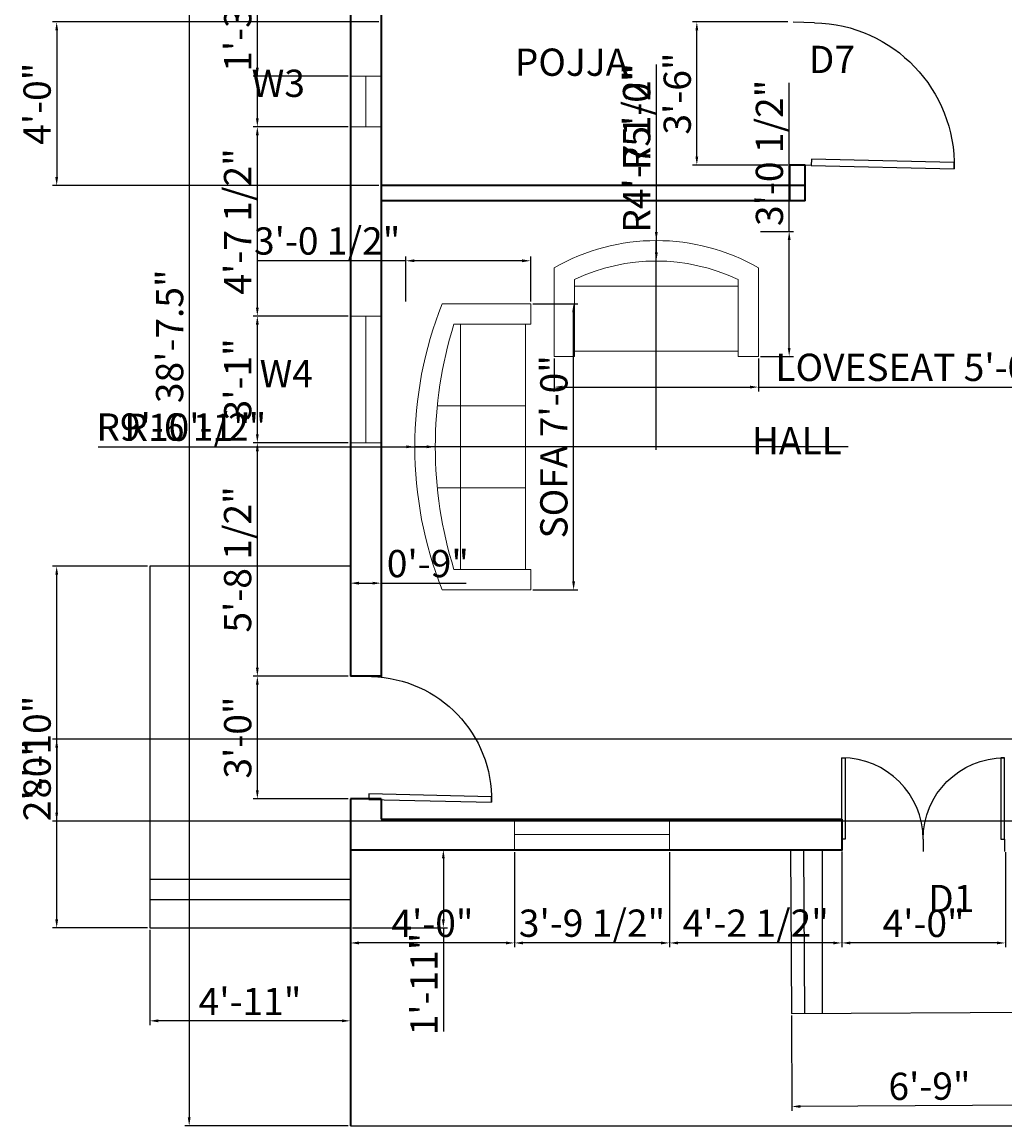
# Model space of a CAD drawing. Units: inches. Extents: x 56 to 631, y 587 to 1198.
# Tile 1 of 3: x 56 to 344, y 622 to 946. Entities that reach past the tile are written whole.
import ezdxf

# ---------------------------------------------------------------- set-up
doc = ezdxf.new("R2010")
doc.units = ezdxf.units.IN
for name, color, linetype, lineweight in [('A-ANNO-DIMS', 2, 'Continuous', 18), ('A-ANNO-TEXT', 7, 'Continuous', 18), ('A-AREA-IDEN', 7, 'Continuous', 25), ('A-DOOR', 3, 'Continuous', 25), ('A-FLOR-OTLN', 7, 'Continuous', 25), ('A-FLOR-STRS', 7, 'Continuous', 25), ('A-FURN', 8, 'Continuous', 18), ('A-GLAZ', 4, 'Continuous', 18), ('WALL', 7, 'Continuous', 35)]:
    doc.layers.add(name, color=color, linetype=linetype, lineweight=lineweight)
doc.styles.get("Standard").update_dxf_attribs({"font": 'arial.ttf', "height": 8})
doc.dimstyles.new('ISO-25', dxfattribs={"dimtxt": 2.5, "dimasz": 2.5, "dimexe": 1.25, "dimexo": 0.625, "dimtad": 1, "dimdec": 1, "dimlunit": 3, "dimtxsty": 'Standard', "dimcen": 2.5, "dimadec": 0, "dimazin": 0, "dimtfac": 1, "dimtdec": 1, "dimtmove": 0, "dimatfit": 3, "dimfxl": 1, "dimarcsym": 0})

# ---------------------------------------------------------------- blocks, each defined once
blk = doc.blocks.new('*U2')
for p, q in [((-40, 0), (-40, 6)), ((0, 0), (0, 6))]:
    blk.add_line(p, q)
blk.add_lwpolyline([(0, 0), (0, -40), (-1.75, -40), (-1.75, 0)], close=True)
blk.add_arc((0, 0), 40, 180, 270)
blk = doc.blocks.new('Sofa - Roundback Loveseat 5 ft.')
for p, q in [((0, -32.44198), (0, -5.99998)), ((-24, -33.99998), (-24, -11.46958)), ((24.00004, -33.99998), (24.00004, -11.46958)), ((-23.9998, -13.38178), (23.99986, -13.38178)), ((-24, -32.44198), (24.00004, -32.44198))]:
    blk.add_line(p, q)
for points in [[(-24, -33.99998), (-30, -33.99998), (-30, -7.99998)], [(30.00004, -7.99998), (30.00004, -33.99998), (24.00004, -33.99998)]]:
    blk.add_lwpolyline(points)
for centre, radius, start, end in [((0, -60.24998), 60.24998, 60.13715, 119.8628), ((0, -61.38438), 55.38444, 64.32083, 115.6792)]:
    blk.add_arc(centre, radius, start, end)
blk = doc.blocks.new('Sofa - Roundback 7 ft.')
for p, q in [((-12.00002, -32.4421), (-12.00003, -6.5971)), ((11.99997, -32.4421), (11.99998, -6.5971)), ((-36.000027, -34), (-36.000027, -11.4696)), ((35.99998, -34), (35.99998, -11.4696)), ((-35.999844, -13.3819), (35.9998, -13.3819)), ((-36.000027, -32.4421), (35.99998, -32.4421))]:
    blk.add_line(p, q)
for points in [[(-36.000027, -34), (-42.000027, -34), (-42.000027, -8)], [(41.99998, -8), (41.99998, -34), (35.99998, -34)]]:
    blk.add_lwpolyline(points)
for centre, radius, start, end in [((0, -114.25), 114.25, 68.43141, 111.5686), ((-0.00001, -127.1968), 121.1968, 72.72033, 107.2797)]:
    blk.add_arc(centre, radius, start, end)
blk = doc.blocks.new('*U3')
for p, q in [((0, 0), (0, -6)), ((40, 0), (40, -6))]:
    blk.add_line(p, q)
blk.add_lwpolyline([(0, 0), (0, 40), (1.75, 40), (1.75, 0)], close=True)
blk.add_arc((0, 0), 40, 0, 90)
blk = doc.blocks.new('*D12')
at = {"layer": 'A-ANNO-DIMS', "color": 0, "lineweight": -2, "transparency": 16777216}
for p, q in [((151.29, 1085.29), (103.37, 1085.29)), ((104.62, 1082.79), (104.62, 624.29)), ((151.29, 621.79), (103.37, 621.79))]:
    blk.add_line(p, q, dxfattribs=at)
at = {"layer": 'A-ANNO-DIMS', "color": 0, "transparency": 16777216}
for points in [[(104.2, 1082.79), (105.03, 1082.79), (104.62, 1085.29)], [(104.2, 624.29), (105.03, 624.29), (104.62, 621.79)]]:
    blk.add_solid(points, dxfattribs=at)
at = {"layer": 'Defpoints', "color": 0, "transparency": 16777216}
for p in [(151.92, 1085.29), (104.62, 621.79), (151.92, 621.79)]:
    blk.add_point(p, dxfattribs=at)
at = {"layer": 'A-ANNO-DIMS', "color": 0, "transparency": 16777216, "insert": (99.9, 853.54), "char_height": 8, "attachment_point": 5, "rotation": 90}
blk.add_mtext('38\'-7.5"', dxfattribs=at)
blk = doc.blocks.new('*D17')
at = {"layer": 'A-ANNO-DIMS', "color": 0, "lineweight": -2, "transparency": 16777216}
for p, q in [((211.72, 847), (211.72, 837.38)), ((271.72, 847), (271.72, 837.38)), ((214.22, 838.63), (269.22, 838.63)), ((271.72, 838.63), (358.5, 838.63))]:
    blk.add_line(p, q, dxfattribs=at)
at = {"layer": 'A-ANNO-DIMS', "color": 0, "transparency": 16777216}
for points in [[(214.22, 839.05), (214.22, 838.21), (211.72, 838.63)], [(269.22, 839.05), (269.22, 838.21), (271.72, 838.63)]]:
    blk.add_solid(points, dxfattribs=at)
at = {"layer": 'Defpoints', "color": 0, "transparency": 16777216}
for p in [(211.72, 847.63), (271.72, 847.63), (271.72, 838.63)]:
    blk.add_point(p, dxfattribs=at)
at = {"layer": 'A-ANNO-DIMS', "color": 0, "transparency": 16777216, "insert": (316.36, 843.39), "char_height": 8, "attachment_point": 5}
blk.add_mtext('LOVESEAT 5\'-0"', dxfattribs=at)
blk = doc.blocks.new('*D18')
at = {"layer": 'A-ANNO-DIMS', "color": 0, "lineweight": -2, "transparency": 16777216}
for p, q in [((280.72, 884.3), (280.72, 927.95)), ((272.35, 884.3), (281.97, 884.3)), ((280.72, 850.13), (280.72, 881.8)), ((272.35, 847.63), (281.97, 847.63))]:
    blk.add_line(p, q, dxfattribs=at)
at = {"layer": 'A-ANNO-DIMS', "color": 0, "transparency": 16777216}
for points in [[(280.31, 881.8), (281.14, 881.8), (280.72, 884.3)], [(280.31, 850.13), (281.14, 850.13), (280.72, 847.63)]]:
    blk.add_solid(points, dxfattribs=at)
at = {"layer": 'Defpoints', "color": 0, "transparency": 16777216}
for p in [(271.72, 884.3), (280.72, 884.3), (271.72, 847.63)]:
    blk.add_point(p, dxfattribs=at)
at = {"layer": 'A-ANNO-DIMS', "color": 0, "transparency": 16777216, "insert": (275.96, 907.37), "char_height": 8, "attachment_point": 5, "rotation": 90}
blk.add_mtext('3\'-0 1/2"', dxfattribs=at)
blk = doc.blocks.new('*D19')
at = {"layer": 'A-ANNO-DIMS', "color": 0, "lineweight": -2, "transparency": 16777216}
for p, q in [((205.48, 863.1), (218.7, 863.1)), ((217.45, 781.6), (217.45, 860.6)), ((205.48, 779.1), (218.7, 779.1))]:
    blk.add_line(p, q, dxfattribs=at)
at = {"layer": 'A-ANNO-DIMS', "color": 0, "transparency": 16777216}
for points in [[(217.03, 860.6), (217.87, 860.6), (217.45, 863.1)], [(217.03, 781.6), (217.87, 781.6), (217.45, 779.1)]]:
    blk.add_solid(points, dxfattribs=at)
at = {"layer": 'Defpoints', "color": 0, "transparency": 16777216}
for p in [(204.85, 863.1), (217.45, 863.1), (204.85, 779.1)]:
    blk.add_point(p, dxfattribs=at)
at = {"layer": 'A-ANNO-DIMS', "color": 0, "transparency": 16777216, "insert": (212.69, 821.1), "char_height": 8, "attachment_point": 5, "rotation": 90}
blk.add_mtext('SOFA 7\'-0"', dxfattribs=at)
blk = doc.blocks.new('*D20')
at = {"layer": 'A-ANNO-DIMS', "color": 0, "lineweight": -2, "transparency": 16777216}
for p, q in [((168.18, 875.7), (124.53, 875.7)), ((168.18, 863.73), (168.18, 876.95)), ((202.35, 875.7), (170.68, 875.7)), ((204.85, 863.73), (204.85, 876.95))]:
    blk.add_line(p, q, dxfattribs=at)
at = {"layer": 'A-ANNO-DIMS', "color": 0, "transparency": 16777216}
for points in [[(170.68, 876.12), (170.68, 875.29), (168.18, 875.7)], [(202.35, 876.12), (202.35, 875.29), (204.85, 875.7)]]:
    blk.add_solid(points, dxfattribs=at)
at = {"layer": 'Defpoints', "color": 0, "transparency": 16777216}
for p in [(168.18, 875.7), (168.18, 863.1), (204.85, 863.1)]:
    blk.add_point(p, dxfattribs=at)
at = {"layer": 'A-ANNO-DIMS', "color": 0, "transparency": 16777216, "insert": (145.11, 880.47), "char_height": 8, "attachment_point": 5, "rotation": 0}
blk.add_mtext('3\'-0 1/2"', dxfattribs=at)
blk = doc.blocks.new('*D21')
at = {"layer": 'A-ANNO-DIMS', "color": 0, "lineweight": -2, "transparency": 16777216}
for p, q in [((93.02, 679.3), (93.02, 651.38)), ((151.92, 679.3), (151.92, 651.38)), ((149.42, 652.63), (95.52, 652.63))]:
    blk.add_line(p, q, dxfattribs=at)
at = {"layer": 'A-ANNO-DIMS', "color": 0, "transparency": 16777216}
for points in [[(95.52, 653.04), (95.52, 652.21), (93.02, 652.63)], [(149.42, 653.04), (149.42, 652.21), (151.92, 652.63)]]:
    blk.add_solid(points, dxfattribs=at)
at = {"layer": 'Defpoints', "color": 0, "transparency": 16777216}
for p in [(93.02, 679.93), (151.92, 679.93), (93.02, 652.63)]:
    blk.add_point(p, dxfattribs=at)
at = {"layer": 'A-ANNO-DIMS', "color": 0, "transparency": 16777216, "insert": (122.47, 657.27), "char_height": 8, "attachment_point": 5}
blk.add_mtext('4\'-11"', dxfattribs=at)
blk = doc.blocks.new('*D28')
at = {"layer": 'A-ANNO-DIMS', "color": 0, "lineweight": -2, "transparency": 16777216}
for p, q in [((160.29, 945.79), (64.47, 945.79)), ((65.72, 943.29), (65.72, 900.29)), ((160.29, 897.79), (64.47, 897.79))]:
    blk.add_line(p, q, dxfattribs=at)
at = {"layer": 'A-ANNO-DIMS', "color": 0, "transparency": 16777216}
for points in [[(65.31, 943.29), (66.14, 943.29), (65.72, 945.79)], [(65.31, 900.29), (66.14, 900.29), (65.72, 897.79)]]:
    blk.add_solid(points, dxfattribs=at)
at = {"layer": 'Defpoints', "color": 0, "transparency": 16777216}
for p in [(160.92, 945.79), (65.72, 897.79), (160.92, 897.79)]:
    blk.add_point(p, dxfattribs=at)
at = {"layer": 'A-ANNO-DIMS', "color": 0, "transparency": 16777216, "insert": (61.01, 921.79), "char_height": 8, "attachment_point": 5, "rotation": 90}
blk.add_mtext('4\'-0"', dxfattribs=at)
blk = doc.blocks.new('*D37')
at = {"layer": 'A-ANNO-DIMS', "color": 0, "lineweight": -2, "transparency": 16777216}
for p, q in [((151.92, 702.16), (151.92, 674.24)), ((200.1, 702.16), (200.1, 674.24)), ((197.6, 675.49), (154.42, 675.49))]:
    blk.add_line(p, q, dxfattribs=at)
at = {"layer": 'A-ANNO-DIMS', "color": 0, "transparency": 16777216}
for points in [[(154.42, 675.9), (154.42, 675.07), (151.92, 675.49)], [(197.6, 675.9), (197.6, 675.07), (200.1, 675.49)]]:
    blk.add_solid(points, dxfattribs=at)
at = {"layer": 'Defpoints', "color": 0, "transparency": 16777216}
for p in [(151.92, 702.79), (200.1, 702.79), (151.92, 675.49)]:
    blk.add_point(p, dxfattribs=at)
at = {"layer": 'A-ANNO-DIMS', "color": 0, "transparency": 16777216, "insert": (176.01, 680.19), "char_height": 8, "attachment_point": 5}
blk.add_mtext('4\'-0"', dxfattribs=at)
blk = doc.blocks.new('*D38')
at = {"layer": 'A-ANNO-DIMS', "color": 0, "lineweight": -2, "transparency": 16777216}
for p, q in [((200.1, 702.16), (200.1, 674.24)), ((245.6, 702.16), (245.6, 674.24)), ((243.1, 675.49), (202.6, 675.49))]:
    blk.add_line(p, q, dxfattribs=at)
at = {"layer": 'A-ANNO-DIMS', "color": 0, "transparency": 16777216}
for points in [[(202.6, 675.9), (202.6, 675.07), (200.1, 675.49)], [(243.1, 675.9), (243.1, 675.07), (245.6, 675.49)]]:
    blk.add_solid(points, dxfattribs=at)
at = {"layer": 'Defpoints', "color": 0, "transparency": 16777216}
for p in [(200.1, 702.79), (245.6, 702.79), (200.1, 675.49)]:
    blk.add_point(p, dxfattribs=at)
at = {"layer": 'A-ANNO-DIMS', "color": 0, "transparency": 16777216, "insert": (222.85, 680.25), "char_height": 8, "attachment_point": 5}
blk.add_mtext('3\'-9 1/2"', dxfattribs=at)
blk = doc.blocks.new('*D39')
at = {"layer": 'A-ANNO-DIMS', "color": 0, "lineweight": -2, "transparency": 16777216}
for p, q in [((245.6, 702.16), (245.6, 674.24)), ((296.18, 702.16), (296.18, 674.24)), ((293.68, 675.49), (248.1, 675.49))]:
    blk.add_line(p, q, dxfattribs=at)
at = {"layer": 'A-ANNO-DIMS', "color": 0, "transparency": 16777216}
for points in [[(248.1, 675.9), (248.1, 675.07), (245.6, 675.49)], [(293.68, 675.9), (293.68, 675.07), (296.18, 675.49)]]:
    blk.add_solid(points, dxfattribs=at)
at = {"layer": 'Defpoints', "color": 0, "transparency": 16777216}
for p in [(245.6, 702.79), (296.18, 702.79), (245.6, 675.49)]:
    blk.add_point(p, dxfattribs=at)
at = {"layer": 'A-ANNO-DIMS', "color": 0, "transparency": 16777216, "insert": (270.89, 680.25), "char_height": 8, "attachment_point": 5}
blk.add_mtext('4\'-2 1/2"', dxfattribs=at)
blk = doc.blocks.new('*D40')
at = {"layer": 'A-ANNO-DIMS', "color": 0, "lineweight": -2, "transparency": 16777216}
for p, q in [((296.18, 702.16), (296.18, 674.24)), ((344.18, 702.16), (344.18, 674.24)), ((341.68, 675.49), (298.68, 675.49))]:
    blk.add_line(p, q, dxfattribs=at)
at = {"layer": 'A-ANNO-DIMS', "color": 0, "transparency": 16777216}
for points in [[(298.68, 675.9), (298.68, 675.07), (296.18, 675.49)], [(341.68, 675.9), (341.68, 675.07), (344.18, 675.49)]]:
    blk.add_solid(points, dxfattribs=at)
at = {"layer": 'Defpoints', "color": 0, "transparency": 16777216}
for p in [(296.18, 702.79), (344.18, 702.79), (296.18, 675.49)]:
    blk.add_point(p, dxfattribs=at)
at = {"layer": 'A-ANNO-DIMS', "color": 0, "transparency": 16777216, "insert": (320.18, 680.19), "char_height": 8, "attachment_point": 5}
blk.add_mtext('4\'-0"', dxfattribs=at)
blk = doc.blocks.new('*D45')
at = {"layer": 'A-ANNO-DIMS', "color": 0, "lineweight": -2, "transparency": 16777216}
for p, q in [((151.29, 1001.7), (123.37, 1001.7)), ((124.62, 932.35), (124.62, 999.2)), ((151.29, 929.85), (123.37, 929.85))]:
    blk.add_line(p, q, dxfattribs=at)
at = {"layer": 'A-ANNO-DIMS', "color": 0, "transparency": 16777216}
for points in [[(124.2, 999.2), (125.03, 999.2), (124.62, 1001.7)], [(124.2, 932.35), (125.03, 932.35), (124.62, 929.85)]]:
    blk.add_solid(points, dxfattribs=at)
at = {"layer": 'Defpoints', "color": 0, "transparency": 16777216}
for p in [(124.62, 1001.7), (151.92, 1001.7), (151.92, 929.85)]:
    blk.add_point(p, dxfattribs=at)
at = {"layer": 'A-ANNO-DIMS', "color": 0, "transparency": 16777216, "insert": (119.91, 965.77), "char_height": 8, "attachment_point": 5, "rotation": 90}
blk.add_mtext('6\'-0"', dxfattribs=at)
blk = doc.blocks.new('*D46')
at = {"layer": 'A-ANNO-DIMS', "color": 0, "lineweight": -2, "transparency": 16777216}
for p, q in [((124.62, 929.85), (124.62, 954.11)), ((151.29, 929.85), (123.37, 929.85)), ((124.62, 917.53), (124.62, 927.35)), ((151.29, 915.03), (123.37, 915.03))]:
    blk.add_line(p, q, dxfattribs=at)
at = {"layer": 'A-ANNO-DIMS', "color": 0, "transparency": 16777216}
for points in [[(124.2, 927.35), (125.03, 927.35), (124.62, 929.85)], [(124.2, 917.53), (125.03, 917.53), (124.62, 915.03)]]:
    blk.add_solid(points, dxfattribs=at)
at = {"layer": 'Defpoints', "color": 0, "transparency": 16777216}
for p in [(124.62, 929.85), (151.92, 929.85), (151.92, 915.03)]:
    blk.add_point(p, dxfattribs=at)
at = {"layer": 'A-ANNO-DIMS', "color": 0, "transparency": 16777216, "insert": (119.9, 943.23), "char_height": 8, "attachment_point": 5, "rotation": 90}
blk.add_mtext('1\'-3"', dxfattribs=at)
blk = doc.blocks.new('*D47')
at = {"layer": 'A-ANNO-DIMS', "color": 0, "lineweight": -2, "transparency": 16777216}
for p, q in [((151.29, 915.03), (123.37, 915.03)), ((124.62, 861.98), (124.62, 912.53)), ((151.29, 859.48), (123.37, 859.48))]:
    blk.add_line(p, q, dxfattribs=at)
at = {"layer": 'A-ANNO-DIMS', "color": 0, "transparency": 16777216}
for points in [[(124.2, 912.53), (125.03, 912.53), (124.62, 915.03)], [(124.2, 861.98), (125.03, 861.98), (124.62, 859.48)]]:
    blk.add_solid(points, dxfattribs=at)
at = {"layer": 'Defpoints', "color": 0, "transparency": 16777216}
for p in [(124.62, 915.03), (151.92, 915.03), (151.92, 859.48)]:
    blk.add_point(p, dxfattribs=at)
at = {"layer": 'A-ANNO-DIMS', "color": 0, "transparency": 16777216, "insert": (119.85, 887.25), "char_height": 8, "attachment_point": 5, "rotation": 90}
blk.add_mtext('4\'-7 1/2"', dxfattribs=at)
blk = doc.blocks.new('*D48')
at = {"layer": 'A-ANNO-DIMS', "color": 0, "lineweight": -2, "transparency": 16777216}
for p, q in [((151.29, 859.48), (123.37, 859.48)), ((124.62, 824.8), (124.62, 856.98)), ((151.29, 822.3), (123.37, 822.3))]:
    blk.add_line(p, q, dxfattribs=at)
at = {"layer": 'A-ANNO-DIMS', "color": 0, "transparency": 16777216}
for points in [[(124.2, 856.98), (125.03, 856.98), (124.62, 859.48)], [(124.2, 824.8), (125.03, 824.8), (124.62, 822.3)]]:
    blk.add_solid(points, dxfattribs=at)
at = {"layer": 'Defpoints', "color": 0, "transparency": 16777216}
for p in [(124.62, 859.48), (151.92, 859.48), (151.92, 822.3)]:
    blk.add_point(p, dxfattribs=at)
at = {"layer": 'A-ANNO-DIMS', "color": 0, "transparency": 16777216, "insert": (119.9, 840.89), "char_height": 8, "attachment_point": 5, "rotation": 90}
blk.add_mtext('3\'-1"', dxfattribs=at)
blk = doc.blocks.new('*D49')
at = {"layer": 'A-ANNO-DIMS', "color": 0, "lineweight": -2, "transparency": 16777216}
for p, q in [((151.29, 822.3), (123.37, 822.3)), ((124.62, 756.28), (124.62, 819.8)), ((151.29, 753.78), (123.37, 753.78))]:
    blk.add_line(p, q, dxfattribs=at)
at = {"layer": 'A-ANNO-DIMS', "color": 0, "transparency": 16777216}
for points in [[(124.2, 819.8), (125.03, 819.8), (124.62, 822.3)], [(124.2, 756.28), (125.03, 756.28), (124.62, 753.78)]]:
    blk.add_solid(points, dxfattribs=at)
at = {"layer": 'Defpoints', "color": 0, "transparency": 16777216}
for p in [(124.62, 822.3), (151.92, 822.3), (151.92, 753.78)]:
    blk.add_point(p, dxfattribs=at)
at = {"layer": 'A-ANNO-DIMS', "color": 0, "transparency": 16777216, "insert": (119.85, 788.04), "char_height": 8, "attachment_point": 5, "rotation": 90}
blk.add_mtext('5\'-8 1/2"', dxfattribs=at)
blk = doc.blocks.new('*D50')
at = {"layer": 'A-ANNO-DIMS', "color": 0, "lineweight": -2, "transparency": 16777216}
for p, q in [((151.29, 753.78), (123.37, 753.78)), ((124.62, 720.28), (124.62, 751.28)), ((151.29, 717.78), (123.37, 717.78))]:
    blk.add_line(p, q, dxfattribs=at)
at = {"layer": 'A-ANNO-DIMS', "color": 0, "transparency": 16777216}
for points in [[(124.2, 751.28), (125.03, 751.28), (124.62, 753.78)], [(124.2, 720.28), (125.03, 720.28), (124.62, 717.78)]]:
    blk.add_solid(points, dxfattribs=at)
at = {"layer": 'Defpoints', "color": 0, "transparency": 16777216}
for p in [(124.62, 753.78), (151.92, 753.78), (151.92, 717.78)]:
    blk.add_point(p, dxfattribs=at)
at = {"layer": 'A-ANNO-DIMS', "color": 0, "transparency": 16777216, "insert": (119.9, 735.78), "char_height": 8, "attachment_point": 5, "rotation": 90}
blk.add_mtext('3\'-0"', dxfattribs=at)
blk = doc.blocks.new('*D60')
at = {"layer": 'A-ANNO-DIMS', "color": 0, "lineweight": -2, "transparency": 16777216}
for p, q in [((280.29, 945.79), (252.37, 945.79)), ((253.62, 906.28), (253.62, 943.29)), ((280.29, 903.78), (252.37, 903.78))]:
    blk.add_line(p, q, dxfattribs=at)
at = {"layer": 'A-ANNO-DIMS', "color": 0, "transparency": 16777216}
for points in [[(253.2, 943.29), (254.03, 943.29), (253.62, 945.79)], [(253.2, 906.28), (254.03, 906.28), (253.62, 903.78)]]:
    blk.add_solid(points, dxfattribs=at)
at = {"layer": 'Defpoints', "color": 0, "transparency": 16777216}
for p in [(253.62, 945.79), (280.92, 945.79), (280.92, 903.78)]:
    blk.add_point(p, dxfattribs=at)
at = {"layer": 'A-ANNO-DIMS', "color": 0, "transparency": 16777216, "insert": (248.9, 924.78), "char_height": 8, "attachment_point": 5, "rotation": 90}
blk.add_mtext('3\'-6"', dxfattribs=at)
blk = doc.blocks.new('*D66')
at = {"layer": 'A-ANNO-DIMS', "color": 0, "lineweight": -2, "transparency": 16777216}
for p, q in [((362.23, 654.59), (362.38, 626.66)), ((281.39, 654.16), (281.53, 626.24)), ((359.87, 627.9), (284.03, 627.5))]:
    blk.add_line(p, q, dxfattribs=at)
at = {"layer": 'A-ANNO-DIMS', "color": 0, "transparency": 16777216}
for points in [[(284.02, 627.92), (284.03, 627.08), (281.53, 627.49)], [(359.87, 628.32), (359.87, 627.48), (362.37, 627.91)]]:
    blk.add_solid(points, dxfattribs=at)
at = {"layer": 'Defpoints', "color": 0, "transparency": 16777216}
for p in [(281.38, 654.79), (362.22, 655.21), (281.53, 627.49)]:
    blk.add_point(p, dxfattribs=at)
at = {"layer": 'A-ANNO-DIMS', "color": 0, "transparency": 16777216, "insert": (321.92, 632.41), "char_height": 8, "attachment_point": 5, "rotation": 0.3029}
blk.add_mtext('6\'-9"', dxfattribs=at)
blk = doc.blocks.new('*D68')
at = {"layer": 'A-ANNO-DIMS', "color": 0, "lineweight": -2, "transparency": 16777216}
for p, q in [((151.92, 754.4), (151.92, 782.33)), ((154.42, 781.08), (158.42, 781.08)), ((160.92, 754.4), (160.92, 782.33)), ((160.92, 781.08), (185.93, 781.08))]:
    blk.add_line(p, q, dxfattribs=at)
at = {"layer": 'A-ANNO-DIMS', "color": 0, "transparency": 16777216}
for points in [[(154.42, 781.49), (154.42, 780.66), (151.92, 781.08)], [(158.42, 781.49), (158.42, 780.66), (160.92, 781.08)]]:
    blk.add_solid(points, dxfattribs=at)
at = {"layer": 'Defpoints', "color": 0, "transparency": 16777216}
for p in [(160.92, 781.08), (151.92, 753.78), (160.92, 753.78)]:
    blk.add_point(p, dxfattribs=at)
at = {"layer": 'A-ANNO-DIMS', "color": 0, "transparency": 16777216, "insert": (174.67, 785.79), "char_height": 8, "attachment_point": 5}
blk.add_mtext('0\'-9"', dxfattribs=at)
blk = doc.blocks.new('*D70')
at = {"layer": 'A-ANNO-DIMS', "color": 0, "lineweight": -2, "transparency": 16777216}
for p, q in [((92.4, 786.03), (64.47, 786.03)), ((65.72, 682.43), (65.72, 783.53)), ((92.4, 679.93), (64.47, 679.93))]:
    blk.add_line(p, q, dxfattribs=at)
at = {"layer": 'A-ANNO-DIMS', "color": 0, "transparency": 16777216}
for points in [[(65.31, 783.53), (66.14, 783.53), (65.72, 786.03)], [(65.31, 682.43), (66.14, 682.43), (65.72, 679.93)]]:
    blk.add_solid(points, dxfattribs=at)
at = {"layer": 'Defpoints', "color": 0, "transparency": 16777216}
for p in [(65.72, 786.03), (93.02, 786.03), (93.02, 679.93)]:
    blk.add_point(p, dxfattribs=at)
at = {"layer": 'A-ANNO-DIMS', "color": 0, "transparency": 16777216, "insert": (61.01, 732.98), "char_height": 8, "attachment_point": 5, "rotation": 90}
blk.add_mtext('8\'-10"', dxfattribs=at)
blk = doc.blocks.new('*D71')
at = {"layer": 'A-ANNO-DIMS', "color": 0, "lineweight": -2, "transparency": 16777216}
for p, q in [((152.54, 702.79), (180.47, 702.79)), ((179.22, 700.29), (179.22, 682.43)), ((152.54, 679.93), (180.47, 679.93)), ((179.22, 679.93), (179.22, 649.45))]:
    blk.add_line(p, q, dxfattribs=at)
at = {"layer": 'A-ANNO-DIMS', "color": 0, "transparency": 16777216}
for points in [[(178.8, 700.29), (179.63, 700.29), (179.22, 702.79)], [(178.8, 682.43), (179.63, 682.43), (179.22, 679.93)]]:
    blk.add_solid(points, dxfattribs=at)
at = {"layer": 'Defpoints', "color": 0, "transparency": 16777216}
for p in [(151.92, 702.79), (151.92, 679.93), (179.22, 679.93)]:
    blk.add_point(p, dxfattribs=at)
at = {"layer": 'A-ANNO-DIMS', "color": 0, "transparency": 16777216, "insert": (174.57, 663.44), "char_height": 8, "attachment_point": 5, "rotation": 90}
blk.add_mtext('1\'-11"', dxfattribs=at)
blk = doc.blocks.new('*D79')
at = {"layer": 'A-ANNO-DIMS', "color": 0, "lineweight": -2, "transparency": 16777216}
for p, q in [((552.89, 735.27), (64.47, 735.27)), ((65.72, 732.77), (65.72, 713.77)), ((557.39, 711.27), (64.47, 711.27))]:
    blk.add_line(p, q, dxfattribs=at)
at = {"layer": 'A-ANNO-DIMS', "color": 0, "transparency": 16777216}
for points in [[(65.31, 732.77), (66.14, 732.77), (65.72, 735.27)], [(65.31, 713.77), (66.14, 713.77), (65.72, 711.27)]]:
    blk.add_solid(points, dxfattribs=at)
at = {"layer": 'Defpoints', "color": 0, "transparency": 16777216}
for p in [(553.52, 735.27), (65.72, 711.27), (558.02, 711.27)]:
    blk.add_point(p, dxfattribs=at)
at = {"layer": 'A-ANNO-DIMS', "color": 0, "transparency": 16777216, "insert": (61.01, 723.27), "char_height": 8, "attachment_point": 5, "rotation": 90}
blk.add_mtext('2\'-0"', dxfattribs=at)
blk = doc.blocks.new('*D81')
at = {"layer": 'A-ANNO-DIMS', "color": 0, "lineweight": -2, "transparency": 16777216}
for p, q in [((85.94, 821.1), (174.35, 821.1)), ((298.05, 821.1), (176.85, 821.1))]:
    blk.add_line(p, q, dxfattribs=at)
at = {"layer": 'A-ANNO-DIMS', "color": 0, "transparency": 16777216}
blk.add_solid([(174.35, 821.52), (174.35, 820.69), (176.85, 821.1)], dxfattribs=at)
at = {"layer": 'Defpoints', "color": 0, "transparency": 16777216}
for p in [(176.85, 821.1), (298.05, 821.1)]:
    blk.add_point(p, dxfattribs=at)
at = {"layer": 'A-ANNO-DIMS', "color": 0, "transparency": 16777216, "insert": (104.13, 825.81), "char_height": 8, "attachment_point": 5}
blk.add_mtext('R10\'-1"', dxfattribs=at)
blk = doc.blocks.new('*D82')
at = {"layer": 'A-ANNO-DIMS', "color": 0, "lineweight": -2, "transparency": 16777216}
for p, q in [((77.89, 821.1), (168.35, 821.1)), ((285.1, 821.1), (170.85, 821.1))]:
    blk.add_line(p, q, dxfattribs=at)
at = {"layer": 'A-ANNO-DIMS', "color": 0, "transparency": 16777216}
blk.add_solid([(168.35, 821.52), (168.35, 820.69), (170.85, 821.1)], dxfattribs=at)
at = {"layer": 'Defpoints', "color": 0, "transparency": 16777216}
for p in [(170.85, 821.1), (285.1, 821.1)]:
    blk.add_point(p, dxfattribs=at)
at = {"layer": 'A-ANNO-DIMS', "color": 0, "transparency": 16777216, "insert": (102.3, 825.86), "char_height": 8, "attachment_point": 5}
blk.add_mtext('R9\'-6 1/2"', dxfattribs=at)
blk = doc.blocks.new('*D83')
at = {"layer": 'A-ANNO-DIMS', "color": 0, "lineweight": -2, "transparency": 16777216}
for p, q in [((241.73, 932.87), (241.73, 884.13)), ((241.72, 821.38), (241.73, 881.63))]:
    blk.add_line(p, q, dxfattribs=at)
at = {"layer": 'A-ANNO-DIMS', "color": 0, "transparency": 16777216}
blk.add_solid([(241.31, 884.13), (242.14, 884.13), (241.73, 881.63)], dxfattribs=at)
at = {"layer": 'Defpoints', "color": 0, "transparency": 16777216}
for p in [(241.73, 881.63), (241.72, 821.38)]:
    blk.add_point(p, dxfattribs=at)
at = {"layer": 'A-ANNO-DIMS', "color": 0, "transparency": 16777216, "insert": (237.02, 917.78), "char_height": 8, "attachment_point": 5, "rotation": 89.9997}
blk.add_mtext('R5\'-0"', dxfattribs=at)
blk = doc.blocks.new('*D84')
at = {"layer": 'A-ANNO-DIMS', "color": 0, "lineweight": -2, "transparency": 16777216}
for p, q in [((241.73, 933.27), (241.73, 878.13)), ((241.72, 820.25), (241.73, 875.63))]:
    blk.add_line(p, q, dxfattribs=at)
at = {"layer": 'A-ANNO-DIMS', "color": 0, "transparency": 16777216}
blk.add_solid([(241.31, 878.13), (242.14, 878.13), (241.73, 875.63)], dxfattribs=at)
at = {"layer": 'Defpoints', "color": 0, "transparency": 16777216}
for p in [(241.73, 875.63), (241.72, 820.25)]:
    blk.add_point(p, dxfattribs=at)
at = {"layer": 'A-ANNO-DIMS', "color": 0, "transparency": 16777216, "insert": (236.96, 908.86), "char_height": 8, "attachment_point": 5, "rotation": 89.9997}
blk.add_mtext('R4\'-7 1/2"', dxfattribs=at)

msp = doc.modelspace()

# ---------------------------------------------------------------- linework, layer by layer
at = {"layer": 'A-FLOR-OTLN'}
msp.add_line((151.92, 621.79), (595.92, 621.79), dxfattribs=at)
at = {"layer": 'A-FLOR-STRS'}
for p, q in [((151.92, 786.03), (93.02, 786.03)), ((93.02, 786.03), (93.02, 786.03)), ((93.02, 786.03), (93.02, 679.93)), ((281.12, 702.79), (281.38, 654.79)), ((284.94, 702.79), (285.19, 654.81)), ((290.49, 654.83), (290.49, 702.79)), ((93.02, 694.23), (151.92, 694.23)), ((93.02, 688.2), (151.92, 688.2)), ((93.02, 679.93), (151.92, 679.93)), ((281.38, 654.79), (362.22, 655.21))]:
    msp.add_line(p, q, dxfattribs=at)
at = {"layer": 'A-GLAZ'}
for p, q in [((151.92, 929.85), (160.92, 929.85)), ((156.42, 929.85), (156.42, 915.03)), ((160.92, 929.85), (160.92, 915.03)), ((160.92, 915.03), (151.92, 915.03)), ((151.92, 859.48), (160.92, 859.48)), ((156.42, 859.48), (156.42, 822.3)), ((160.92, 859.48), (160.92, 822.3)), ((160.92, 822.3), (151.92, 822.3)), ((200.1, 711.79), (200.1, 702.79)), ((245.6, 702.79), (245.6, 711.79)), ((200.1, 707.29), (245.6, 707.29)), ((200.1, 702.79), (245.6, 702.79))]:
    msp.add_line(p, q, dxfattribs=at)
at = {"layer": 'WALL'}
for p, q in [((151.92, 1085.29), (151.92, 753.78)), ((160.92, 1076.29), (160.92, 753.78)), ((280.92, 893.29), (280.92, 903.78)), ((285.37, 903.78), (280.92, 903.78)), ((285.42, 897.79), (285.37, 903.78)), ((285.42, 897.79), (160.92, 897.79)), ((285.42, 893.29), (285.42, 897.79)), ((285.42, 893.29), (160.92, 893.29)), ((161.22, 753.78), (151.92, 753.78)), ((160.92, 717.78), (151.92, 717.78)), ((151.92, 717.78), (151.92, 621.79)), ((160.92, 717.78), (160.92, 711.79)), ((160.92, 711.79), (296.18, 711.79)), ((280.92, 711.79), (296.18, 711.79)), ((296.18, 711.79), (296.18, 702.79)), ((151.92, 702.79), (296.18, 702.79))]:
    msp.add_line(p, q, dxfattribs=at)

# ---------------------------------------------------------------- block references
at = {"layer": 'A-DOOR', "rotation": 88.70842365487967}
for p, xscale, yscale, zscale in [((287.21, 903.64), -1.048793395041371, 1.048793395041371, 1.048793395041371), ((157.35, 717.63), -0.9005162739509557, 0.9005162739509559, 0.9005162739509559)]:
    msp.add_blockref('*U2', p, dxfattribs=dict(at, xscale=xscale, yscale=yscale, zscale=zscale))
at = {"layer": 'A-DOOR', "yscale": 0.5971299030301838, "zscale": 0.5971299030301838}
for p, xscale in [((296.15, 705.95), 0.5971299030301838), ((343.92, 705.95), -0.5971299030301838)]:
    msp.add_blockref('*U3', p, dxfattribs=dict(at, xscale=xscale))
at = {"layer": 'A-FURN'}
msp.add_blockref('Sofa - Roundback Loveseat 5 ft.', (241.72, 881.63), dxfattribs=at)
at = {"layer": 'A-FURN', "rotation": 90.00001645868946}
msp.add_blockref('Sofa - Roundback 7 ft.', (170.85, 821.1), dxfattribs=at)

# ---------------------------------------------------------------- texts
at = {"layer": 'A-ANNO-TEXT'}
for s, p in [('D7', (286.48, 930.79)), ('W3', (122.95, 923.79)), ('W4', (125.29, 838.59)), ('D1', (321.52, 684.54))]:
    msp.add_text(s, height=8, dxfattribs=at).set_placement(p)
at = {"layer": 'A-AREA-IDEN'}
for s, p in [('POJJA', (200.18, 929.98)), ('HALL', (269.76, 818.89))]:
    msp.add_text(s, height=8, dxfattribs=at).set_placement(p)

# ---------------------------------------------------------------- dimensions: what is measured, and where the dimension line sits
at = {"layer": 'A-ANNO-DIMS'}
for base, p1, p2, angle, override, picture, middle in [((104.62, 621.79), (151.92, 1085.29), (151.92, 621.79), 90, {"dimclrd": 0, "dimclre": 0, "dimclrt": 0}, '*D12', (99.9, 853.54)), ((124.6152, 1001.6956), (151.9152, 929.8485), (151.9152, 1001.6956), 90, {"dimdec": 1, "dimlfac": 1, "dimrnd": 0, "dimzin": 1, "dimdsep": 46, "dimlunit": 4, "dimfrac": 2}, '*D45', (119.9057, 965.7721)), ((124.62, 929.85), (151.92, 915.03), (151.92, 929.85), 90, {"dimdec": 1, "dimlfac": 1, "dimrnd": 0, "dimzin": 1, "dimdsep": 46, "dimlunit": 4, "dimfrac": 2}, '*D46', (119.9, 943.23)), ((65.72, 897.79), (160.92, 945.79), (160.92, 897.79), 90, {"dimdec": 1, "dimlfac": 1, "dimrnd": 0, "dimzin": 1, "dimdsep": 46, "dimlunit": 4, "dimfrac": 2}, '*D28', (61.01, 921.79)), ((253.62, 945.79), (280.92, 903.78), (280.92, 945.79), 90, {"dimdec": 1, "dimlfac": 1, "dimrnd": 0, "dimzin": 1, "dimdsep": 46, "dimlunit": 4, "dimfrac": 2}, '*D60', (248.9, 924.78)), ((280.72, 884.3), (271.72, 847.63), (271.72, 884.3), 90, {"dimdec": 1, "dimlfac": 1, "dimrnd": 0, "dimzin": 1, "dimdsep": 46, "dimlunit": 4, "dimfrac": 2}, '*D18', (275.96, 907.37)), ((124.6152, 915.0312), (151.9152, 859.4763), (151.9152, 915.0312), 90, {"dimdec": 1, "dimlfac": 1, "dimrnd": 0, "dimzin": 1, "dimdsep": 46, "dimlunit": 4, "dimfrac": 2}, '*D47', (119.8538, 887.2538)), ((168.18, 875.7), (204.85, 863.1), (168.18, 863.1), 180, {"dimdec": 1, "dimlfac": 1, "dimrnd": 0, "dimzin": 1, "dimdsep": 46, "dimlunit": 4, "dimfrac": 2}, '*D20', (145.11, 880.47)), ((124.62, 859.48), (151.92, 822.3), (151.92, 859.48), 90, {"dimdec": 1, "dimlfac": 1, "dimrnd": 0, "dimzin": 1, "dimdsep": 46, "dimlunit": 4, "dimfrac": 2}, '*D48', (119.9, 840.89)), ((124.62, 822.3), (151.92, 753.78), (151.92, 822.3), 90, {"dimdec": 1, "dimlfac": 1, "dimrnd": 0, "dimzin": 1, "dimdsep": 46, "dimlunit": 4, "dimfrac": 2}, '*D49', (119.85, 788.04)), ((65.72, 786.03), (93.02, 679.93), (93.02, 786.03), 90, {"dimdec": 1, "dimlfac": 1, "dimrnd": 0, "dimzin": 1, "dimdsep": 46, "dimlunit": 4, "dimfrac": 2}, '*D70', (61.01, 732.98)), ((124.62, 753.78), (151.92, 717.78), (151.92, 753.78), 90, {"dimdec": 1, "dimlfac": 1, "dimrnd": 0, "dimzin": 1, "dimdsep": 46, "dimlunit": 4, "dimfrac": 2}, '*D50', (119.9, 735.78)), ((65.72, 711.27), (553.52, 735.27), (558.02, 711.27), 90, {"dimdec": 1, "dimlfac": 1, "dimrnd": 0, "dimzin": 1, "dimdsep": 46, "dimlunit": 4, "dimfrac": 2}, '*D79', (61.01, 723.27)), ((151.92, 675.49), (200.1, 702.79), (151.92, 702.79), 180, {"dimdec": 1, "dimlfac": 1, "dimrnd": 0, "dimzin": 1, "dimdsep": 46, "dimlunit": 4, "dimfrac": 2}, '*D37', (176.01, 680.19)), ((179.22, 679.93), (151.92, 702.79), (151.92, 679.93), 270, {"dimdec": 1, "dimlfac": 1, "dimrnd": 0, "dimzin": 1, "dimdsep": 46, "dimlunit": 4, "dimfrac": 2}, '*D71', (174.57, 663.44)), ((200.1, 675.49), (245.6, 702.79), (200.1, 702.79), 180, {"dimdec": 1, "dimlfac": 1, "dimrnd": 0, "dimzin": 1, "dimdsep": 46, "dimlunit": 4, "dimfrac": 2}, '*D38', (222.85, 680.25)), ((245.6, 675.49), (296.18, 702.79), (245.6, 702.79), 180, {"dimdec": 1, "dimlfac": 1, "dimrnd": 0, "dimzin": 1, "dimdsep": 46, "dimlunit": 4, "dimfrac": 2}, '*D39', (270.89, 680.25)), ((296.18, 675.49), (344.18, 702.79), (296.18, 702.79), 180, {"dimdec": 1, "dimlfac": 1, "dimrnd": 0, "dimzin": 1, "dimdsep": 46, "dimlunit": 4, "dimfrac": 2}, '*D40', (320.18, 680.19)), ((93.02, 652.63), (151.92, 679.93), (93.02, 679.93), 180, {"dimdec": 1, "dimlfac": 1, "dimrnd": 0, "dimzin": 1, "dimdsep": 46, "dimlunit": 4, "dimfrac": 2}, '*D21', (122.47, 657.27)), ((281.53, 627.49), (362.22, 655.21), (281.38, 654.79), 180.3029, {"dimdec": 1, "dimlfac": 1, "dimrnd": 0, "dimzin": 1, "dimdsep": 46, "dimlunit": 4, "dimfrac": 2}, '*D66', (321.92, 632.41))]:
    dim = msp.add_linear_dim(base=base, p1=p1, p2=p2, angle=angle, dimstyle='ISO-25', override=override, dxfattribs=at)
    dim.commit()
    dim.dimension.update_dxf_attribs({"geometry": picture, "text_midpoint": middle})
for center, mpoint, picture, middle in [((241.72, 820.25), (241.73, 875.63), '*D84', (241.73, 908.86)), ((241.7247, 821.3799), (241.725, 881.6298), '*D83', (241.7252, 917.7798)), ((285.100747, 821.103104), (170.850747, 821.103), '*D82', (102.300747, 821.103)), ((298.05, 821.1), (176.85, 821.1), '*D81', (104.13, 821.1))]:
    dim = msp.add_radius_dim(center=center, mpoint=mpoint, dimstyle='ISO-25', override={"dimdec": 1, "dimlfac": 1, "dimrnd": 0, "dimzin": 1, "dimdsep": 46, "dimlunit": 4, "dimfrac": 2}, dxfattribs=at)
    dim.commit()
    dim.dimension.update_dxf_attribs({"geometry": picture, "text_midpoint": middle, "dimtype": 164})
dim = msp.add_linear_dim(base=(217.45, 863.1), p1=(204.85, 779.1), p2=(204.85, 863.1), angle=90, text='SOFA <>', dimstyle='ISO-25', override={"dimdec": 1, "dimlfac": 1, "dimrnd": 0, "dimzin": 1, "dimdsep": 46, "dimlunit": 4, "dimfrac": 2}, dxfattribs=at)
dim.commit()
dim.dimension.update_dxf_attribs({"geometry": '*D19', "text_midpoint": (212.69, 821.1)})
dim = msp.add_linear_dim(base=(271.72, 838.63), p1=(211.72, 847.63), p2=(271.72, 847.63), text='LOVESEAT <>', dimstyle='ISO-25', override={"dimdec": 1, "dimlfac": 1, "dimrnd": 0, "dimzin": 1, "dimdsep": 46, "dimlunit": 4, "dimfrac": 2}, dxfattribs=at)
dim.commit()
dim.dimension.update_dxf_attribs({"geometry": '*D17', "text_midpoint": (316.36, 843.39)})
dim = msp.add_linear_dim(base=(160.92, 781.08), p1=(151.92, 753.78), p2=(160.92, 753.78), dimstyle='ISO-25', override={"dimdec": 1, "dimlfac": 1, "dimrnd": 0, "dimzin": 1, "dimdsep": 46, "dimlunit": 4, "dimfrac": 2}, dxfattribs=at)
dim.commit()
dim.dimension.update_dxf_attribs({"geometry": '*D68', "text_midpoint": (174.67, 785.79)})

doc.saveas('drawing.dxf')
